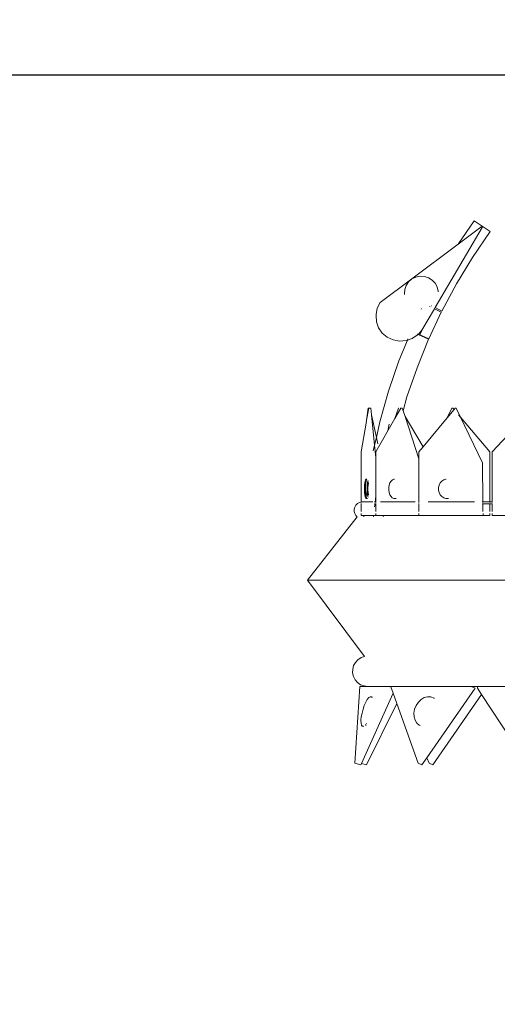
# Model space of a CAD drawing. Units: millimetres. Extents: x 7894 to 8038, y 6851 to 6951.
# Tile 10 of 49: x 7974.616 to 7976.35, y 6875.21 to 6878.784. Entities that reach past the tile are written whole.
import ezdxf

# ---------------------------------------------------------------- set-up
doc = ezdxf.new("R2010")
doc.units = ezdxf.units.MM
for name, color, linetype, lineweight in [('A-ANNO-DIMS', 2, 'Continuous', 18), ('A-FURN-ACCS', 8, 'Continuous', 13), ('A-FURN-SHLF', 7, 'Continuous', 30)]:
    doc.layers.add(name, color=color, linetype=linetype, lineweight=lineweight)
doc.styles.get("Standard").update_dxf_attribs({"font": 'arial.ttf'})
doc.dimstyles.new('ISO-25', dxfattribs={"dimtxt": 1, "dimasz": 1, "dimexe": 1.25, "dimexo": 0.625, "dimtad": 1, "dimdec": 0, "dimlunit": 4, "dimtxsty": 'Standard', "dimcen": 2.5, "dimclrt": 1, "dimadec": 0, "dimazin": 0, "dimtfac": 1, "dimtdec": 0, "dimtmove": 0, "dimatfit": 3, "dimfxl": 1, "dimarcsym": 0})

# ---------------------------------------------------------------- blocks, each defined once
blk = doc.blocks.new('*D36')
at = {"layer": 'A-ANNO-DIMS', "color": 0, "lineweight": -2, "transparency": 16777216}
for p, q in [((7980.8359, 6877.9586), (7980.8359, 6858.5122)), ((7944.4866, 6864.4359), (7944.4866, 6858.5122)), ((7945.4866, 6859.7622), (7979.8359, 6859.7622))]:
    blk.add_line(p, q, dxfattribs=at)
at = {"layer": 'A-ANNO-DIMS', "color": 0, "transparency": 16777216}
for points in [[(7945.4866, 6859.9288), (7945.4866, 6859.5955), (7944.4866, 6859.7622)], [(7979.8359, 6859.9288), (7979.8359, 6859.5955), (7980.8359, 6859.7622)]]:
    blk.add_solid(points, dxfattribs=at)
at = {"layer": 'Defpoints', "color": 0, "transparency": 16777216}
for p in [(7980.8359, 6878.5836), (7944.4866, 6865.0609), (7980.8359, 6859.7622)]:
    blk.add_point(p, dxfattribs=at)
at = {"layer": 'A-ANNO-DIMS', "color": 1, "transparency": 16777216, "insert": (7962.6613, 6860.9046), "char_height": 1, "attachment_point": 5}
blk.add_mtext('3\'-0 1/2"', dxfattribs=at)
blk = doc.blocks.new('*D39')
at = {"layer": 'A-ANNO-DIMS', "color": 0, "lineweight": -2, "transparency": 16777216}
for p, q in [((7982.6834, 6874.8578), (7982.6834, 6879.7661)), ((7964.1574, 6873.8578), (7983.9334, 6873.8578)), ((7982.6834, 6872.9028), (7982.6834, 6873.8578)), ((7981.4609, 6872.9028), (7983.9334, 6872.9028)), ((7982.6834, 6871.9028), (7982.6834, 6870.9028))]:
    blk.add_line(p, q, dxfattribs=at)
at = {"layer": 'A-ANNO-DIMS', "color": 0, "transparency": 16777216}
for points in [[(7982.5168, 6874.8578), (7982.8501, 6874.8578), (7982.6834, 6873.8578)], [(7982.5168, 6871.9028), (7982.8501, 6871.9028), (7982.6834, 6872.9028)]]:
    blk.add_solid(points, dxfattribs=at)
at = {"layer": 'Defpoints', "color": 0, "transparency": 16777216}
for p in [(7963.5324, 6873.8578), (7982.6834, 6873.8578), (7980.8359, 6872.9028)]:
    blk.add_point(p, dxfattribs=at)
at = {"layer": 'A-ANNO-DIMS', "color": 1, "transparency": 16777216, "insert": (7981.5479, 6877.8119), "char_height": 1, "attachment_point": 5, "rotation": 90}
blk.add_mtext('0\'-1"', dxfattribs=at)
blk = doc.blocks.new('*D40')
at = {"layer": 'A-ANNO-DIMS', "color": 0, "lineweight": -2, "transparency": 16777216}
for p, q in [((7982.6834, 6878.5836), (7982.6834, 6885.822)), ((7981.4609, 6878.5836), (7983.9334, 6878.5836)), ((7982.6834, 6874.8578), (7982.6834, 6877.5836)), ((7964.1574, 6873.8578), (7983.9334, 6873.8578))]:
    blk.add_line(p, q, dxfattribs=at)
at = {"layer": 'A-ANNO-DIMS', "color": 0, "transparency": 16777216}
for points in [[(7982.5168, 6877.5836), (7982.8501, 6877.5836), (7982.6834, 6878.5836)], [(7982.5168, 6874.8578), (7982.8501, 6874.8578), (7982.6834, 6873.8578)]]:
    blk.add_solid(points, dxfattribs=at)
at = {"layer": 'Defpoints', "color": 0, "transparency": 16777216}
for p in [(7980.8359, 6878.5836), (7982.6834, 6878.5836), (7963.5324, 6873.8578)]:
    blk.add_point(p, dxfattribs=at)
at = {"layer": 'A-ANNO-DIMS', "color": 1, "transparency": 16777216, "insert": (7981.5414, 6882.7028), "char_height": 1, "attachment_point": 5, "rotation": 90}
blk.add_mtext('0\'-4 1/2"', dxfattribs=at)

msp = doc.modelspace()

# ---------------------------------------------------------------- linework, layer by layer
at = {"layer": 'A-FURN-ACCS'}
for p, q in [((7976.2655, 6878.0544, 2.197), (7976.2074, 6877.9696, 2.197)), ((7976.2944, 6878.0346, 2.197), (7976.2655, 6878.0544, 2.197)), ((7976.2944, 6878.0301, 2.197), (7976.1236, 6877.7389, 2.197)), ((7976.2944, 6878.0346, 2.197), (7976.2074, 6877.9696, 2.197)), ((7976.2944, 6878.0301, 2.197), (7976.2944, 6878.0346, 2.197)), ((7976.3232, 6878.0149, 2.197), (7976.2944, 6878.0346, 2.197)), ((7976.2593, 6877.9215, 2.197), (7976.3232, 6878.0149, 2.197)), ((7976.2074, 6877.9696, 2.197), (7976.0393, 6877.843, 2.197)), ((7976.2009, 6877.8256, 2.197), (7976.2593, 6877.9215, 2.197)), ((7976.0393, 6877.843, 2.197), (7975.9241, 6877.7575, 2.197)), ((7976.0274, 6877.8326, 2.197), (7976.0393, 6877.843, 2.197)), ((7976.0393, 6877.843, 2.197), (7976.0535, 6877.85, 2.197)), ((7976.0535, 6877.85, 2.197), (7976.0692, 6877.8532, 2.197)), ((7976.0692, 6877.8532, 2.197), (7976.0851, 6877.8523, 2.197)), ((7976.0851, 6877.8523, 2.197), (7976.1003, 6877.8476, 2.197)), ((7976.1003, 6877.8476, 2.197), (7976.1137, 6877.8392, 2.197)), ((7976.1137, 6877.8392, 2.197), (7976.1244, 6877.8277, 2.197)), ((7976.013, 6877.7896, 2.197), (7976.0138, 6877.805, 2.197)), ((7976.0138, 6877.805, 2.197), (7976.0187, 6877.8197, 2.197)), ((7976.0187, 6877.8197, 2.197), (7976.0274, 6877.8326, 2.197)), ((7976.1244, 6877.8277, 2.197), (7976.1316, 6877.814, 2.197)), ((7976.1316, 6877.814, 2.197), (7976.1349, 6877.7989, 2.197)), ((7976.2009, 6877.8256, 2.197), (7976.1479, 6877.7267, 2.197)), ((7976.0131, 6877.7891, 2.197), (7976.013, 6877.7896, 2.197)), ((7976.013, 6877.7869, 2.197), (7976.0131, 6877.7891, 2.197)), ((7976.1348, 6877.7967, 2.197), (7976.1349, 6877.7989, 2.197)), ((7976.1348, 6877.7967, 2.197), (7976.1349, 6877.7962, 2.197)), ((7975.9138, 6877.7369, 2.197), (7975.9094, 6877.7145, 2.197)), ((7975.9241, 6877.7575, 2.197), (7975.9138, 6877.7369, 2.197)), ((7976.0748, 6877.7355, 2.197), (7976.0736, 6877.7329, 2.197)), ((7976.1212, 6877.7347, 2.197), (7976.0756, 6877.657, 2.197)), ((7976.1035, 6877.743, 2.197), (7976.1063, 6877.7417, 2.197)), ((7976.1112, 6877.7451, 2.197), (7976.1092, 6877.7461, 2.197)), ((7976.1236, 6877.7389, 2.197), (7976.1212, 6877.7347, 2.197)), ((7976.1461, 6877.723, 2.197), (7976.1212, 6877.7347, 2.197)), ((7976.1236, 6877.7389, 2.197), (7976.1479, 6877.7267, 2.197)), ((7975.9094, 6877.71, 2.197), (7975.9094, 6877.7145, 2.197)), ((7975.9094, 6877.71, 2.197), (7975.9111, 6877.6872, 2.197)), ((7976.1005, 6877.6258, 2.197), (7976.1461, 6877.723, 2.197)), ((7975.9111, 6877.6872, 2.197), (7975.9189, 6877.6656, 2.197)), ((7975.9189, 6877.6656, 2.197), (7975.9322, 6877.6467, 2.197)), ((7976.0806, 6877.6655, 2.197), (7976.0689, 6877.6406, 2.197)), ((7975.9322, 6877.6467, 2.197), (7975.9501, 6877.6318, 2.197)), ((7975.9501, 6877.6318, 2.197), (7975.9714, 6877.6219, 2.197)), ((7976.0231, 6877.621, 2.197), (7976.0406, 6877.6268, 2.197)), ((7976.0253, 6877.6262, 2.197), (7976.0231, 6877.621, 2.197)), ((7976.0406, 6877.6268, 2.197), (7976.0601, 6877.6397, 2.197)), ((7976.0581, 6877.521, 2.197), (7976.1002, 6877.6251, 2.197)), ((7976.0586, 6877.6432, 2.197), (7976.062, 6877.6417, 2.197)), ((7976.0601, 6877.6397, 2.197), (7976.062, 6877.6417, 2.197)), ((7976.0633, 6877.6432, 2.197), (7976.0607, 6877.6444, 2.197)), ((7976.062, 6877.6417, 2.197), (7976.0633, 6877.6432, 2.197)), ((7976.062, 6877.6417, 2.197), (7976.1002, 6877.6251, 2.197)), ((7976.0633, 6877.6432, 2.197), (7976.0756, 6877.657, 2.197)), ((7976.0633, 6877.6432, 2.197), (7976.1005, 6877.6258, 2.197)), ((7976.0689, 6877.6406, 2.197), (7976.0682, 6877.639, 2.197)), ((7975.9714, 6877.6219, 2.197), (7975.9947, 6877.6176, 2.197)), ((7976.0231, 6877.621, 2.197), (7975.9926, 6877.5455, 2.197)), ((7975.9947, 6877.6176, 2.197), (7976.0182, 6877.6193, 2.197)), ((7976.0182, 6877.6193, 2.197), (7976.0231, 6877.621, 2.197)), ((7975.9926, 6877.5455, 2.197), (7975.955, 6877.4357, 2.197)), ((7976.0217, 6877.4148, 2.197), (7976.0581, 6877.521, 2.197)), ((7975.955, 6877.4357, 2.197), (7975.9233, 6877.3241, 2.197)), ((7976.0076, 6877.3649, 2.197), (7976.0217, 6877.4148, 2.197)), ((7975.875, 6877.331, 2.197), (7975.8805, 6877.3745, 2.197)), ((7975.8834, 6877.3745, 2.197), (7975.875, 6877.331, 2.197)), ((7975.8834, 6877.3745, 2.197), (7975.8805, 6877.3745, 2.197)), ((7975.8834, 6877.3745, 2.197), (7975.8902, 6877.3745, 2.197)), ((7975.8928, 6877.3496, 2.197), (7975.8902, 6877.3745, 2.197)), ((7975.9774, 6877.3369, 2.197), (7975.9905, 6877.3745, 2.197)), ((7975.9988, 6877.3745, 2.197), (7975.9774, 6877.3369, 2.197)), ((7975.9921, 6877.3745, 2.197), (7975.9905, 6877.3745, 2.197)), ((7976.0044, 6877.3745, 2.197), (7975.9988, 6877.3745, 2.197)), ((7976.0076, 6877.3649, 2.197), (7976.0044, 6877.3745, 2.197)), ((7976.1676, 6877.3393, 2.197), (7976.185, 6877.3745, 2.197)), ((7976.188, 6877.3745, 2.197), (7976.185, 6877.3745, 2.197)), ((7976.188, 6877.3745, 2.197), (7976.1925, 6877.3693, 2.197)), ((7976.1969, 6877.3745, 2.197), (7976.1925, 6877.3693, 2.197)), ((7976.2002, 6877.3745, 2.197), (7976.1969, 6877.3745, 2.197)), ((7976.2162, 6877.3414, 2.197), (7976.2002, 6877.3745, 2.197)), ((7975.8928, 6877.3496, 2.197), (7975.9107, 6877.2681, 2.197)), ((7975.9042, 6877.2395, 2.197), (7975.8928, 6877.3496, 2.197)), ((7976.0147, 6877.3433, 2.197), (7976.0076, 6877.3649, 2.197)), ((7976.0147, 6877.3433, 2.197), (7976.0801, 6877.2342, 2.197)), ((7976.0648, 6877.1907, 2.197), (7976.0147, 6877.3433, 2.197)), ((7976.1676, 6877.3393, 2.197), (7976.0801, 6877.2342, 2.197)), ((7976.1925, 6877.3693, 2.197), (7976.1676, 6877.3393, 2.197)), ((7976.2085, 6877.3504, 2.197), (7976.2162, 6877.3414, 2.197)), ((7976.2162, 6877.3414, 2.197), (7976.3231, 6877.2159, 2.197)), ((7976.2964, 6877.1753, 2.197), (7976.2162, 6877.3414, 2.197)), ((7975.8736, 6877.3201, 2.197), (7975.855, 6877.2159, 2.197)), ((7975.8736, 6877.3201, 2.197), (7975.875, 6877.331, 2.197)), ((7975.9774, 6877.3369, 2.197), (7975.9088, 6877.2159, 2.197)), ((7975.9233, 6877.3241, 2.197), (7975.9107, 6877.2681, 2.197)), ((7975.9572, 6877.3155, 2.197), (7975.9519, 6877.2918, 2.197)), ((7976.4254, 6877.3158, 2.197), (7976.3309, 6877.2159, 2.197)), ((7975.9107, 6877.2681, 2.197), (7975.9042, 6877.2395, 2.197)), ((7975.9107, 6877.2681, 2.197), (7975.9159, 6877.2445, 2.197)), ((7975.9042, 6877.2395, 2.197), (7975.8995, 6877.2187, 2.197)), ((7975.9088, 6877.1954, 2.197), (7975.9042, 6877.2395, 2.197)), ((7976.0801, 6877.2342, 2.197), (7976.0648, 6877.2159, 2.197)), ((7975.855, 6877.2159, 2.197), (7975.8555, 6877.1778, 2.197)), ((7975.9088, 6877.2159, 2.197), (7975.9088, 6877.1954, 2.197)), ((7975.9088, 6877.1954, 2.197), (7975.9088, 6877.0335, 2.197)), ((7976.0648, 6877.2159, 2.197), (7976.0648, 6877.1907, 2.197)), ((7976.3231, 6877.2159, 2.197), (7976.3231, 6877.0335, 2.197)), ((7976.3309, 6877.2159, 2.197), (7976.3309, 6877.0335, 2.197)), ((7975.8552, 6877.1753, 2.197), (7975.8549, 6877.033, 2.197)), ((7975.8552, 6877.1753, 2.197), (7975.8555, 6877.1778, 2.197)), ((7976.0648, 6877.1907, 2.197), (7976.0648, 6877.0315, 2.197)), ((7976.2964, 6877.1753, 2.197), (7976.2974, 6877.0335, 2.197)), ((7975.8673, 6877.086, 2.197), (7975.8677, 6877.0948, 2.197)), ((7975.8677, 6877.0948, 2.197), (7975.8686, 6877.1027, 2.197)), ((7975.8686, 6877.1027, 2.197), (7975.8698, 6877.1091, 2.197)), ((7975.8698, 6877.1091, 2.197), (7975.8713, 6877.1137, 2.197)), ((7975.8707, 6877.086, 2.197), (7975.8711, 6877.0948, 2.197)), ((7975.8711, 6877.0948, 2.197), (7975.872, 6877.1027, 2.197)), ((7975.8713, 6877.1137, 2.197), (7975.873, 6877.116, 2.197)), ((7975.872, 6877.1027, 2.197), (7975.8732, 6877.1091, 2.197)), ((7975.8764, 6877.116, 2.197), (7975.873, 6877.116, 2.197)), ((7975.8732, 6877.1091, 2.197), (7975.8747, 6877.1137, 2.197)), ((7975.8747, 6877.1137, 2.197), (7975.8764, 6877.116, 2.197)), ((7975.8772, 6877.0946, 2.197), (7975.8766, 6877.0858, 2.197)), ((7975.8782, 6877.1025, 2.197), (7975.8772, 6877.0946, 2.197)), ((7975.8784, 6877.0965, 2.197), (7975.8772, 6877.0946, 2.197)), ((7975.8797, 6877.109, 2.197), (7975.8782, 6877.1025, 2.197)), ((7975.8782, 6877.1025, 2.197), (7975.8784, 6877.0965, 2.197)), ((7975.8806, 6877.1112, 2.197), (7975.8797, 6877.109, 2.197)), ((7975.8808, 6877.1106, 2.197), (7975.8797, 6877.109, 2.197)), ((7975.8806, 6877.0946, 2.197), (7975.88, 6877.0858, 2.197)), ((7975.8816, 6877.1025, 2.197), (7975.8806, 6877.0946, 2.197)), ((7975.8821, 6877.1046, 2.197), (7975.8816, 6877.1025, 2.197)), ((7975.9558, 6877.086, 2.197), (7975.9572, 6877.0948, 2.197)), ((7975.9572, 6877.0948, 2.197), (7975.96, 6877.1027, 2.197)), ((7975.96, 6877.1027, 2.197), (7975.9639, 6877.1091, 2.197)), ((7975.9639, 6877.1091, 2.197), (7975.9686, 6877.1137, 2.197)), ((7975.9686, 6877.1137, 2.197), (7975.9739, 6877.116, 2.197)), ((7975.9767, 6877.116, 2.197), (7975.9739, 6877.116, 2.197)), ((7976.1363, 6877.086, 2.197), (7976.1384, 6877.0948, 2.197)), ((7976.1384, 6877.0948, 2.197), (7976.1424, 6877.1027, 2.197)), ((7976.1424, 6877.1027, 2.197), (7976.1481, 6877.1091, 2.197)), ((7976.1481, 6877.1091, 2.197), (7976.155, 6877.1137, 2.197)), ((7976.155, 6877.1137, 2.197), (7976.1628, 6877.116, 2.197)), ((7976.1645, 6877.116, 2.197), (7976.1628, 6877.116, 2.197)), ((7975.8673, 6877.0769, 2.197), (7975.8673, 6877.086, 2.197)), ((7975.8677, 6877.0681, 2.197), (7975.8673, 6877.0769, 2.197)), ((7975.8686, 6877.0601, 2.197), (7975.8677, 6877.0681, 2.197)), ((7975.8698, 6877.0537, 2.197), (7975.8686, 6877.0601, 2.197)), ((7975.8713, 6877.0491, 2.197), (7975.8698, 6877.0537, 2.197)), ((7975.8707, 6877.0769, 2.197), (7975.8707, 6877.086, 2.197)), ((7975.8711, 6877.0681, 2.197), (7975.8707, 6877.0769, 2.197)), ((7975.872, 6877.0601, 2.197), (7975.8711, 6877.0681, 2.197)), ((7975.8732, 6877.0537, 2.197), (7975.872, 6877.0601, 2.197)), ((7975.8766, 6877.0767, 2.197), (7975.8732, 6877.0537, 2.197)), ((7975.8747, 6877.0491, 2.197), (7975.8732, 6877.0537, 2.197)), ((7975.8766, 6877.0858, 2.197), (7975.8766, 6877.0767, 2.197)), ((7975.8766, 6877.0767, 2.197), (7975.8772, 6877.0679, 2.197)), ((7975.8772, 6877.0679, 2.197), (7975.8782, 6877.06, 2.197)), ((7975.8782, 6877.06, 2.197), (7975.8797, 6877.0536, 2.197)), ((7975.8797, 6877.0536, 2.197), (7975.8806, 6877.0515, 2.197)), ((7975.88, 6877.0858, 2.197), (7975.88, 6877.0767, 2.197)), ((7975.88, 6877.0767, 2.197), (7975.8806, 6877.0679, 2.197)), ((7975.8806, 6877.0679, 2.197), (7975.8816, 6877.06, 2.197)), ((7975.8816, 6877.06, 2.197), (7975.8821, 6877.058, 2.197)), ((7975.9088, 6877.0552, 2.197), (7975.9061, 6877.0315, 2.197)), ((7975.9558, 6877.0769, 2.197), (7975.9558, 6877.086, 2.197)), ((7975.9572, 6877.0681, 2.197), (7975.9558, 6877.0769, 2.197)), ((7975.9599, 6877.0601, 2.197), (7975.9572, 6877.0681, 2.197)), ((7975.9638, 6877.0537, 2.197), (7975.9599, 6877.0601, 2.197)), ((7975.9685, 6877.0491, 2.197), (7975.9638, 6877.0537, 2.197)), ((7976.1362, 6877.0769, 2.197), (7976.1363, 6877.086, 2.197)), ((7976.1383, 6877.0681, 2.197), (7976.1362, 6877.0769, 2.197)), ((7976.1423, 6877.0601, 2.197), (7976.1383, 6877.0681, 2.197)), ((7976.1479, 6877.0537, 2.197), (7976.1423, 6877.0601, 2.197)), ((7976.1549, 6877.0491, 2.197), (7976.1479, 6877.0537, 2.197)), ((7975.8322, 6877.0152, 2.197), (7975.8363, 6877.0221, 2.197)), ((7975.8363, 6877.0221, 2.197), (7975.842, 6877.0276, 2.197)), ((7975.842, 6877.0276, 2.197), (7975.849, 6877.0315, 2.197)), ((7975.849, 6877.0315, 2.197), (7975.8549, 6877.033, 2.197)), ((7975.8549, 6877.033, 2.197), (7975.8567, 6877.0335, 2.197)), ((7975.8549, 6877.033, 2.197), (7975.8549, 6877.0315, 2.197)), ((7975.8549, 6877.0276, 2.197), (7975.8549, 6876.9995, 2.197)), ((7975.8567, 6877.0335, 2.197), (7975.8581, 6877.0335, 2.197)), ((7975.8567, 6877.0335, 2.197), (7975.8573, 6877.0335, 2.197)), ((7975.8977, 6877.0335, 2.197), (7975.8581, 6877.0335, 2.197)), ((7975.8729, 6877.0467, 2.197), (7975.8713, 6877.0491, 2.197)), ((7975.8747, 6877.0467, 2.197), (7975.8729, 6877.0467, 2.197)), ((7975.8764, 6877.0467, 2.197), (7975.8747, 6877.0491, 2.197)), ((7975.8764, 6877.0467, 2.197), (7975.8747, 6877.0467, 2.197)), ((7975.8781, 6877.0467, 2.197), (7975.8764, 6877.0467, 2.197)), ((7975.9088, 6877.0335, 2.197), (7975.9043, 6877.0335, 2.197)), ((7975.9057, 6877.0276, 2.197), (7975.9043, 6877.0157, 2.197)), ((7975.9088, 6877.0271, 2.197), (7975.9043, 6877.0271, 2.197)), ((7975.9088, 6877.0335, 2.197), (7975.9088, 6877.0315, 2.197)), ((7975.9088, 6877.0276, 2.197), (7975.9088, 6877.0271, 2.197)), ((7975.9088, 6877.0271, 2.197), (7975.9088, 6876.9995, 2.197)), ((7976.0516, 6877.0335, 2.197), (7975.9254, 6877.0335, 2.197)), ((7975.9738, 6877.0467, 2.197), (7975.9685, 6877.0491, 2.197)), ((7975.9793, 6877.0467, 2.197), (7975.9738, 6877.0467, 2.197)), ((7975.9821, 6877.0467, 2.197), (7975.9793, 6877.0467, 2.197)), ((7976.0648, 6877.0276, 2.197), (7976.0648, 6876.9995, 2.197)), ((7976.0989, 6877.0335, 2.197), (7976.2669, 6877.0335, 2.197)), ((7976.1626, 6877.0467, 2.197), (7976.1549, 6877.0491, 2.197)), ((7976.1707, 6877.0467, 2.197), (7976.1626, 6877.0467, 2.197)), ((7976.1723, 6877.0467, 2.197), (7976.1707, 6877.0467, 2.197)), ((7976.2974, 6877.0335, 2.197), (7976.2941, 6877.0335, 2.197)), ((7976.2975, 6877.0271, 2.197), (7976.2942, 6877.0271, 2.197)), ((7976.2974, 6877.0335, 2.197), (7976.2975, 6877.0315, 2.197)), ((7976.3231, 6877.0335, 2.197), (7976.2974, 6877.0335, 2.197)), ((7976.2975, 6877.0276, 2.197), (7976.2975, 6877.0271, 2.197)), ((7976.2975, 6877.0271, 2.197), (7976.2977, 6876.9995, 2.197)), ((7976.3231, 6877.0271, 2.197), (7976.2975, 6877.0271, 2.197)), ((7976.3231, 6877.0335, 2.197), (7976.3309, 6877.0335, 2.197)), ((7976.3231, 6877.0335, 2.197), (7976.3231, 6877.0315, 2.197)), ((7976.3231, 6877.0276, 2.197), (7976.3231, 6877.0271, 2.197)), ((7976.3231, 6877.0271, 2.197), (7976.3231, 6876.9995, 2.197)), ((7976.3309, 6877.0271, 2.197), (7976.3231, 6877.0271, 2.197)), ((7976.3309, 6877.0335, 2.197), (7976.3309, 6877.0315, 2.197)), ((7976.3309, 6877.0276, 2.197), (7976.3309, 6877.0271, 2.197)), ((7976.3309, 6877.0271, 2.197), (7976.3309, 6876.9995, 2.197)), ((7975.8299, 6876.9995, 2.197), (7975.83, 6877.0075, 2.197)), ((7975.8319, 6876.9918, 2.197), (7975.8299, 6876.9995, 2.197)), ((7975.83, 6877.0075, 2.197), (7975.8322, 6877.0152, 2.197)), ((7975.8358, 6876.9848, 2.197), (7975.8319, 6876.9918, 2.197)), ((7975.8413, 6876.9791, 2.197), (7975.8358, 6876.9848, 2.197)), ((7975.8549, 6876.9918, 2.197), (7975.8548, 6876.9848, 2.197)), ((7975.8555, 6876.9848, 2.197), (7975.8548, 6876.9848, 2.197)), ((7975.8656, 6876.9848, 2.197), (7975.8548, 6876.9848, 2.197)), ((7975.8652, 6876.9813, 2.197), (7975.865, 6876.9791, 2.197)), ((7975.8656, 6876.9848, 2.197), (7975.8652, 6876.9813, 2.197)), ((7975.9088, 6876.9848, 2.197), (7975.8656, 6876.9848, 2.197)), ((7975.9008, 6876.9848, 2.197), (7975.9001, 6876.9791, 2.197)), ((7975.9088, 6876.9918, 2.197), (7975.9088, 6876.9848, 2.197)), ((7975.9088, 6876.9848, 2.197), (7975.936, 6876.9848, 2.197)), ((7975.9353, 6876.9791, 2.197), (7975.936, 6876.9848, 2.197)), ((7975.936, 6876.9848, 2.197), (7976.0652, 6876.9848, 2.197)), ((7976.0648, 6876.9918, 2.197), (7976.0652, 6876.9848, 2.197)), ((7976.0652, 6876.9848, 2.197), (7976.2978, 6876.9848, 2.197)), ((7976.2978, 6876.9918, 2.197), (7976.2978, 6876.9848, 2.197)), ((7976.3231, 6876.9848, 2.197), (7976.2978, 6876.9848, 2.197)), ((7976.3231, 6876.9918, 2.197), (7976.3231, 6876.9848, 2.197)), ((7976.3309, 6876.9918, 2.197), (7976.3309, 6876.9848, 2.197)), ((7976.3309, 6876.9848, 2.197), (7976.592, 6876.9848, 2.197)), ((7975.6603, 6876.7501, 2.197), (7975.8413, 6876.9791, 2.197)), ((7975.8675, 6876.4729, 2.197), (7975.6603, 6876.7501, 2.197)), ((7977.2625, 6876.7501, 2.197), (7975.6603, 6876.7501, 2.197)), ((7975.8281, 6876.4395, 2.197), (7975.8346, 6876.4513, 2.197)), ((7975.8346, 6876.4513, 2.197), (7975.8437, 6876.4611, 2.197)), ((7975.8437, 6876.4611, 2.197), (7975.8549, 6876.4685, 2.197)), ((7975.8549, 6876.4685, 2.197), (7975.8675, 6876.4729, 2.197)), ((7975.8245, 6876.4132, 2.197), (7975.8247, 6876.4266, 2.197)), ((7975.8275, 6876.4001, 2.197), (7975.8245, 6876.4132, 2.197)), ((7975.8247, 6876.4266, 2.197), (7975.8281, 6876.4395, 2.197)), ((7975.8336, 6876.3882, 2.197), (7975.8275, 6876.4001, 2.197)), ((7975.8424, 6876.3781, 2.197), (7975.8336, 6876.3882, 2.197)), ((7975.8534, 6876.3704, 2.197), (7975.8424, 6876.3781, 2.197)), ((7975.8318, 6876.0853, 2.197), (7975.8511, 6876.364, 2.197)), ((7975.8793, 6876.364, 2.197), (7975.8511, 6876.364, 2.197)), ((7975.866, 6876.3656, 2.197), (7975.8534, 6876.3704, 2.197)), ((7975.8568, 6876.0843, 2.197), (7975.9712, 6876.3398, 2.197)), ((7975.8793, 6876.364, 2.197), (7975.866, 6876.3656, 2.197)), ((7975.8793, 6876.364, 2.197), (7975.9573, 6876.364, 2.197)), ((7975.9573, 6876.364, 2.197), (7975.9626, 6876.364, 2.197)), ((7975.9633, 6876.3621, 2.197), (7975.9573, 6876.364, 2.197)), ((7975.9633, 6876.3621, 2.197), (7975.9626, 6876.364, 2.197)), ((7975.9626, 6876.364, 2.197), (7976.2547, 6876.364, 2.197)), ((7975.9712, 6876.3398, 2.197), (7975.9633, 6876.3621, 2.197)), ((7975.9848, 6876.3017, 2.197), (7975.9712, 6876.3398, 2.197)), ((7976.0943, 6876.1052, 2.197), (7976.269, 6876.3576, 2.197)), ((7976.2547, 6876.364, 2.197), (7976.2778, 6876.364, 2.197)), ((7976.269, 6876.3576, 2.197), (7976.2547, 6876.364, 2.197)), ((7976.2778, 6876.3576, 2.197), (7976.2778, 6876.364, 2.197)), ((7976.6121, 6876.364, 2.197), (7976.2778, 6876.364, 2.197)), ((7976.2926, 6876.335, 2.197), (7976.2778, 6876.3576, 2.197)), ((7975.8668, 6876.295, 2.197), (7975.8721, 6876.3071, 2.197)), ((7975.8721, 6876.3071, 2.197), (7975.8776, 6876.3167, 2.197)), ((7975.8751, 6876.079, 2.197), (7975.9848, 6876.3017, 2.197)), ((7975.8776, 6876.3167, 2.197), (7975.8831, 6876.3234, 2.197)), ((7975.8831, 6876.3234, 2.197), (7975.888, 6876.3267, 2.197)), ((7975.888, 6876.3267, 2.197), (7975.8921, 6876.3263, 2.197)), ((7975.8928, 6876.3254, 2.197), (7975.8921, 6876.3263, 2.197)), ((7975.8928, 6876.3254, 2.197), (7975.8969, 6876.325, 2.197)), ((7976.0619, 6876.0853, 2.197), (7975.9848, 6876.3017, 2.197)), ((7976.0551, 6876.295, 2.197), (7976.0632, 6876.3071, 2.197)), ((7976.0632, 6876.3071, 2.197), (7976.0732, 6876.3167, 2.197)), ((7976.0732, 6876.3167, 2.197), (7976.0845, 6876.3234, 2.197)), ((7976.0845, 6876.3234, 2.197), (7976.0963, 6876.3267, 2.197)), ((7976.0963, 6876.3267, 2.197), (7976.1079, 6876.3263, 2.197)), ((7976.1079, 6876.3263, 2.197), (7976.1187, 6876.322, 2.197)), ((7976.1154, 6876.079, 2.197), (7976.2926, 6876.335, 2.197)), ((7976.1187, 6876.322, 2.197), (7976.1214, 6876.3209, 2.197)), ((7976.402, 6876.1672, 2.197), (7976.2926, 6876.335, 2.197)), ((7975.8559, 6876.2537, 2.197), (7975.8584, 6876.2674, 2.197)), ((7975.8584, 6876.2674, 2.197), (7975.8622, 6876.2815, 2.197)), ((7975.8622, 6876.2815, 2.197), (7975.8668, 6876.295, 2.197)), ((7976.047, 6876.2674, 2.197), (7976.0496, 6876.2815, 2.197)), ((7976.0475, 6876.2537, 2.197), (7976.047, 6876.2674, 2.197)), ((7976.0496, 6876.2815, 2.197), (7976.0551, 6876.295, 2.197)), ((7975.8547, 6876.2413, 2.197), (7975.8559, 6876.2537, 2.197)), ((7975.8549, 6876.2311, 2.197), (7975.8547, 6876.2413, 2.197)), ((7975.8566, 6876.2237, 2.197), (7975.8549, 6876.2311, 2.197)), ((7976.051, 6876.2413, 2.197), (7976.0475, 6876.2537, 2.197)), ((7976.0573, 6876.2311, 2.197), (7976.051, 6876.2413, 2.197)), ((7976.066, 6876.2237, 2.197), (7976.0573, 6876.2311, 2.197)), ((7975.8596, 6876.2196, 2.197), (7975.8566, 6876.2237, 2.197)), ((7975.8637, 6876.2193, 2.197), (7975.8596, 6876.2196, 2.197)), ((7975.8644, 6876.2183, 2.197), (7975.8637, 6876.2193, 2.197)), ((7975.8715, 6876.2261, 2.197), (7975.8733, 6876.2225, 2.197)), ((7975.8733, 6876.2225, 2.197), (7975.8741, 6876.2219, 2.197)), ((7975.8745, 6876.23, 2.197), (7975.8748, 6876.2278, 2.197)), ((7976.069, 6876.2223, 2.197), (7976.066, 6876.2237, 2.197)), ((7976.0762, 6876.079, 2.197), (7976.0943, 6876.1052, 2.197)), ((7976.1024, 6876.0853, 2.197), (7976.0943, 6876.1052, 2.197)), ((7975.8544, 6876.079, 2.197), (7975.8318, 6876.0853, 2.197)), ((7975.8544, 6876.079, 2.197), (7975.8568, 6876.0843, 2.197)), ((7975.8751, 6876.079, 2.197), (7975.8568, 6876.0843, 2.197)), ((7976.0762, 6876.079, 2.197), (7976.0619, 6876.0853, 2.197)), ((7976.1154, 6876.079, 2.197), (7976.1024, 6876.0853, 2.197))]:
    msp.add_line(p, q, dxfattribs=at)
at = {"layer": 'A-FURN-SHLF'}
msp.add_line((7963.5324, 6878.5836, -3.5), (7980.8359, 6878.5836, -3.5), dxfattribs=at)

# ---------------------------------------------------------------- dimensions: what is measured, and where the dimension line sits
at = {"layer": 'A-ANNO-DIMS'}
for base, p1, p2, picture, middle in [((7982.6834, 6878.5836), (7963.5324, 6873.8578), (7980.8359, 6878.5836), '*D40', (7981.5414, 6882.7028)), ((7982.6834, 6873.8578), (7980.8359, 6872.9028), (7963.5324, 6873.8578), '*D39', (7981.5479, 6877.8119))]:
    dim = msp.add_linear_dim(base=base, p1=p1, p2=p2, angle=90, dimstyle='ISO-25', override={"dimdec": 1, "dimlfac": 1, "dimrnd": 0, "dimzin": 1, "dimdsep": 46, "dimlunit": 4, "dimfrac": 2}, dxfattribs=at)
    dim.commit()
    dim.dimension.update_dxf_attribs({"geometry": picture, "text_midpoint": middle})
dim = msp.add_linear_dim(base=(7980.8359, 6859.7622), p1=(7944.4866, 6865.0609), p2=(7980.8359, 6878.5836), dimstyle='ISO-25', override={"dimdec": 1, "dimlfac": 1, "dimrnd": 0, "dimzin": 1, "dimdsep": 46, "dimlunit": 4, "dimfrac": 2}, dxfattribs=at)
dim.commit()
dim.dimension.update_dxf_attribs({"geometry": '*D36', "text_midpoint": (7962.6613, 6860.9046)})

doc.saveas('drawing.dxf')
